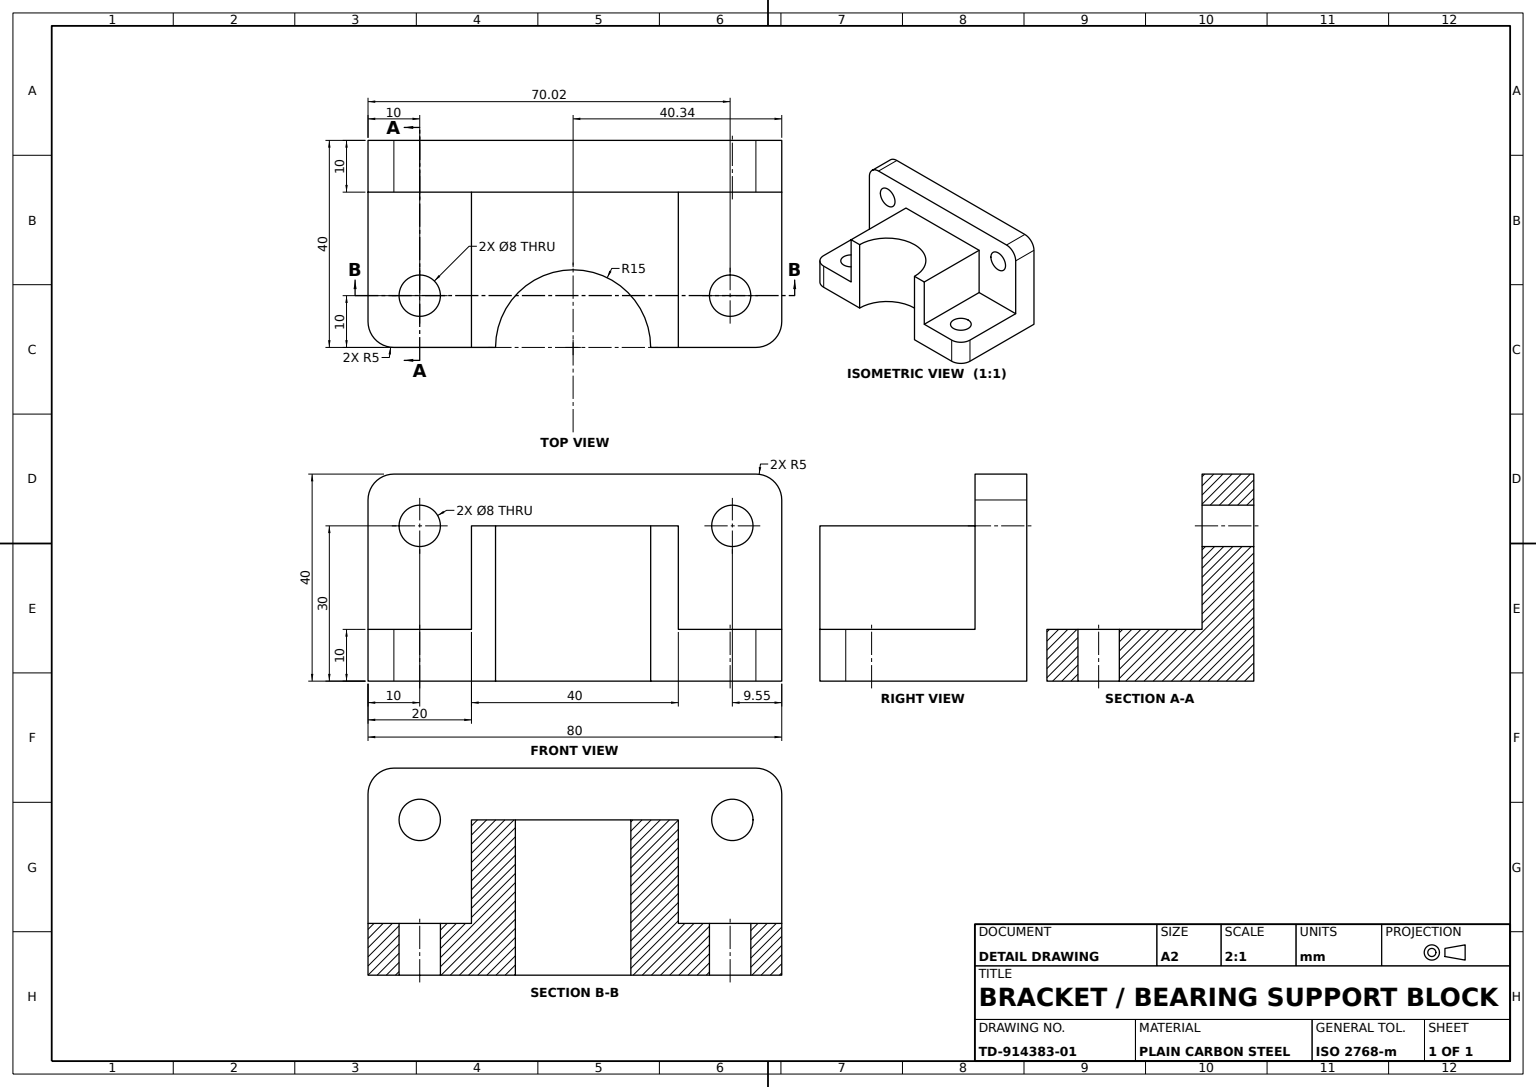
SolidWorks part; units mm, degrees
material "Plain Carbon Steel"
ref_plane "Front Plane" through (0, 0, 0) normal (0, 0, 1) x (1, 0, 0)
ref_plane "Top Plane" through (0, 0, 0) normal (0, 1, 0) x (1, 0, 0)
ref_plane "Right Plane" through (0, 0, 0) normal (1, 0, 0) x (0, 0, -1)
sketch "Back Plate Sketch" plane through (0, 0, 0) normal (0, 0, 1) x (1, 0, 0)
  line L3 (0, 0) -> (80, 0)
  line L6 (0, 0) -> (0, 35)
  line L7 (80, 0) -> (80, 35)
  line L10 (5, 40) -> (75, 40)
  arc A3 (5, 40) -> (0, 35) centre (5, 35) ccw
  arc A4 (80, 35) -> (75, 40) centre (75, 35) ccw
  dimension "D1" = 10
  dimension "D2" = 10
  dimension "D3" = 40
  dimension "D5" = 5
  dimension "D6" = 80
  dimension "D4" = 35
extrude "Back Plate" add sketch "Back Plate Sketch" along normal blind 10
sketch "Base Plate Sketch" plane through (0, 0, 0) normal (0, -1, 0) x (1, 0, 0)
  line L0 (0, 10) -> (0, 35)
  line L1 (80, 10) -> (80, 35)
  line L2 (0, 10) -> (20, 10)
  line L3 (80, 10) -> (80, 0) construction
  line L4 (0, 10) -> (80, 10) construction
  line L7 (5, 40) -> (20, 40)
  line L9 (20, 10) -> (20, 40)
  line L10 (60, 10) -> (80, 10)
  line L11 (60, 10) -> (60, 40)
  line L12 (60, 40) -> (75, 40)
  line L13 (0, 0) -> (80, 0) construction
  arc A0 (5, 40) -> (0, 35) centre (5, 35) ccw
  arc A1 (80, 35) -> (75, 40) centre (75, 35) ccw
  dimension "D1" = 10
  dimension "D2" = 10
  dimension "D3" = 5
  dimension "D4" = 20
  dimension "D5" = 40
extrude "Base Plate" add sketch "Base Plate Sketch" against normal blind 10
sketch "Bearing Block Sketch" plane through (0, 0, 0) normal (0, -1, 0) x (1, 0, 0)
  line L0 (20, 10) -> (20, 40)
  line L1 (80, 35) -> (80, 0) construction
  line L2 (20, 40) -> (24.656, 40)
  line L3 (60, 10) -> (60, 40)
  line L4 (60, 40) -> (54.656, 40)
  line L5 (20, 10) -> (60, 10)
  arc A0 (24.656, 40) -> (54.656, 40) centre (39.656, 40) ccw
  dimension "D1" = 30
  dimension "D2" = 15
  dimension "D3" = 40.344
extrude "Bearing Block" add sketch "Bearing Block Sketch" against normal blind 30
sketch "Back Plate Holes Sketch" plane through (0, 0, 10) normal (0, 0, 1) x (1, 0, 0)
  line L0 (75, 40) -> (5, 40) construction
  line L1 (0, 35) -> (0, 10) construction
  line L2 (80, 10) -> (80, 35) construction
  circle A0 centre (10, 30) radius 4
  circle A1 centre (70.4472, 30) radius 4
  dimension "D1" = 8
  dimension "D4" = 8
  dimension "D5" = 8
  dimension "D2" = 10
  dimension "D3" = 10
  dimension "D6" = 9.5528
extrude "Back Plate Holes 2xØ8" cut sketch "Back Plate Holes Sketch" against normal blind 10
sketch "Base Plate Holes Sketch" plane through (0, 10, 0) normal (0, 1, 0) x (1, 0, 0)
  line L0 (20, -40) -> (5, -40) construction
  line L1 (0, -35) -> (0, -10) construction
  circle A0 centre (10, -30) radius 4
  circle A1 centre (70.0171, -30) radius 4
  dimension "D1" = 8
  dimension "D4" = 8
  dimension "D5" = 8
  dimension "D2" = 10
  dimension "D3" = 10
  dimension "D6" = 70.0171
extrude "Base Plate Holes 2xØ8" cut sketch "Base Plate Holes Sketch" against normal blind 10
